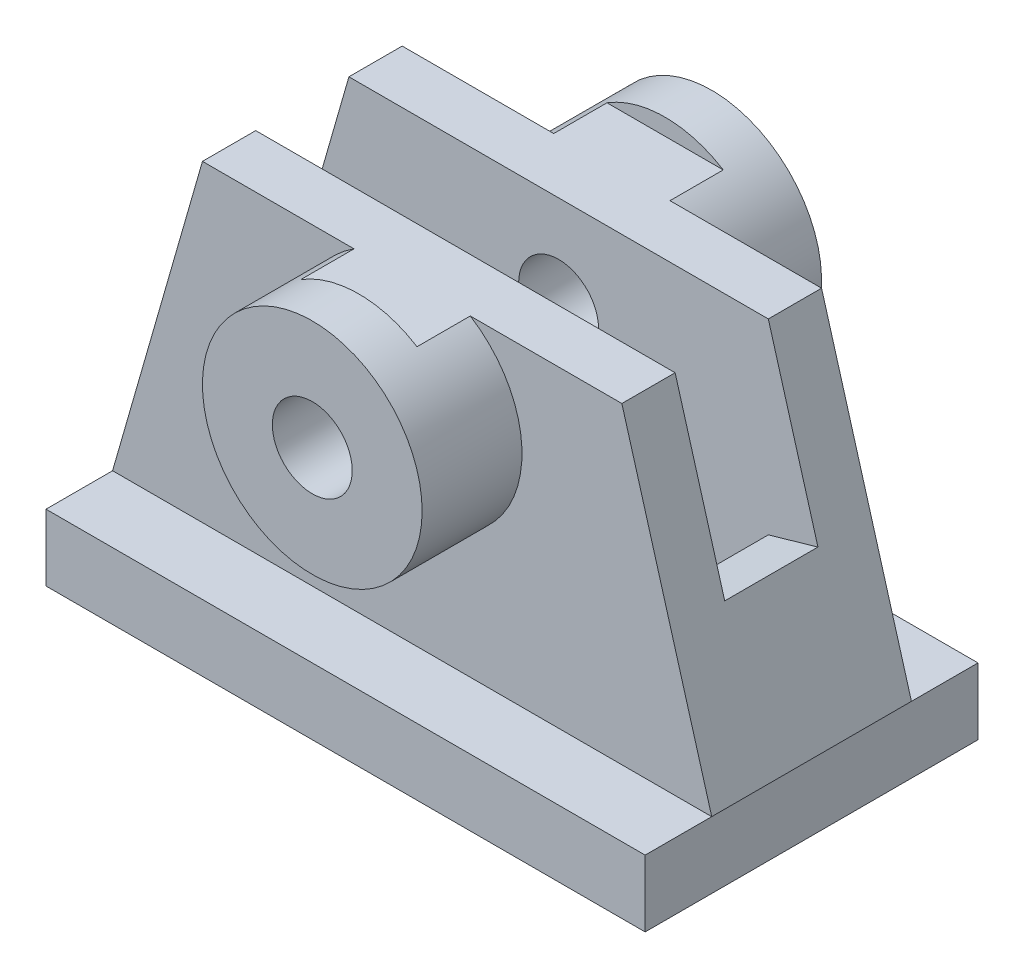
ISO-10303-21;
HEADER;
FILE_DESCRIPTION(('STEP AP214'),'2;1');
FILE_NAME('part.step','',(''),(''),'','','');
FILE_SCHEMA(('AUTOMOTIVE_DESIGN { 1 0 10303 214 1 1 1 1 }'));
ENDSEC;
DATA;
#1=APPLICATION_CONTEXT('core data for automotive mechanical design processes');
#2=APPLICATION_PROTOCOL_DEFINITION('international standard','automotive_design',2000,#1);
#3=PRODUCT_CONTEXT('',#1,'mechanical');
#4=PRODUCT('Part','Part','',(#3));
#5=PRODUCT_RELATED_PRODUCT_CATEGORY('part','',(#4));
#6=PRODUCT_DEFINITION_FORMATION('','',#4);
#7=PRODUCT_DEFINITION_CONTEXT('part definition',#1,'design');
#8=PRODUCT_DEFINITION('design','',#6,#7);
#9=PRODUCT_DEFINITION_SHAPE('','',#8);
#10=(LENGTH_UNIT() NAMED_UNIT(*) SI_UNIT(.MILLI.,.METRE.));
#11=(NAMED_UNIT(*) PLANE_ANGLE_UNIT() SI_UNIT($,.RADIAN.));
#12=(NAMED_UNIT(*) SI_UNIT($,.STERADIAN.) SOLID_ANGLE_UNIT());
#13=UNCERTAINTY_MEASURE_WITH_UNIT(LENGTH_MEASURE(1.E-05),#10,'distance_accuracy_value','');
#14=(GEOMETRIC_REPRESENTATION_CONTEXT(3) GLOBAL_UNCERTAINTY_ASSIGNED_CONTEXT((#13)) GLOBAL_UNIT_ASSIGNED_CONTEXT((#10,
#11,#12)) REPRESENTATION_CONTEXT('',''));
#15=CARTESIAN_POINT('',(0.,0.,0.));
#16=DIRECTION('',(0.,0.,1.));
#17=DIRECTION('',(1.,0.,0.));
#18=AXIS2_PLACEMENT_3D('',#15,#16,#17);
#19=CARTESIAN_POINT('',(0.,43.,-30.));
#20=DIRECTION('',(0.,0.,1.));
#21=DIRECTION('',(1.,0.,0.));
#22=AXIS2_PLACEMENT_3D('',#19,#20,#21);
#23=CYLINDRICAL_SURFACE('',#22,16.5);
#24=CARTESIAN_POINT('',(0.,43.,-30.));
#25=DIRECTION('',(0.,0.,-1.));
#26=DIRECTION('',(-1.,0.,0.));
#27=AXIS2_PLACEMENT_3D('',#24,#25,#26);
#28=CIRCLE('',#27,16.5);
#29=CARTESIAN_POINT('',(-16.5,43.,-30.));
#30=VERTEX_POINT('',#29);
#31=EDGE_CURVE('E334',#30,#30,#28,.T.);
#32=ORIENTED_EDGE('',*,*,#31,.F.);
#33=EDGE_LOOP('',(#32));
#34=FACE_BOUND('',#33,.T.);
#35=DIRECTION('',(0.,0.,-1.));
#36=VECTOR('',#35,1.);
#37=CARTESIAN_POINT('',(-8.73212459828648,57.,195.564259305483));
#38=LINE('',#37,#36);
#39=CARTESIAN_POINT('',(-8.73212459828648,57.,-15.));
#40=VERTEX_POINT('',#39);
#41=CARTESIAN_POINT('',(-8.73212459828648,57.,-23.));
#42=VERTEX_POINT('',#41);
#43=EDGE_CURVE('E177',#40,#42,#38,.T.);
#44=ORIENTED_EDGE('',*,*,#43,.T.);
#45=CARTESIAN_POINT('',(0.,43.,-23.));
#46=DIRECTION('',(0.,0.,-1.));
#47=DIRECTION('',(-1.,0.,0.));
#48=AXIS2_PLACEMENT_3D('',#45,#46,#47);
#49=CIRCLE('',#48,16.5);
#50=CARTESIAN_POINT('',(8.73212459828648,57.,-23.));
#51=VERTEX_POINT('',#50);
#52=EDGE_CURVE('E350',#42,#51,#49,.T.);
#53=ORIENTED_EDGE('',*,*,#52,.T.);
#54=DIRECTION('',(0.,0.,-1.));
#55=VECTOR('',#54,1.);
#56=CARTESIAN_POINT('',(8.73212459828648,57.,195.564259305483));
#57=LINE('',#56,#55);
#58=CARTESIAN_POINT('',(8.73212459828648,57.,-15.));
#59=VERTEX_POINT('',#58);
#60=EDGE_CURVE('E53',#59,#51,#57,.T.);
#61=ORIENTED_EDGE('',*,*,#60,.F.);
#62=CARTESIAN_POINT('',(0.,43.,-15.));
#63=DIRECTION('',(0.,0.,-1.));
#64=DIRECTION('',(-1.,0.,0.));
#65=AXIS2_PLACEMENT_3D('',#62,#63,#64);
#66=CIRCLE('',#65,16.5);
#67=EDGE_CURVE('E50',#40,#59,#66,.F.);
#68=ORIENTED_EDGE('',*,*,#67,.F.);
#69=EDGE_LOOP('',(#44,#53,#61,#68));
#70=FACE_BOUND('',#69,.T.);
#71=ADVANCED_FACE('F39',(#34,#70),#23,.T.);
#72=CARTESIAN_POINT('',(0.,43.,30.));
#73=DIRECTION('',(0.,0.,-1.));
#74=DIRECTION('',(-1.,0.,0.));
#75=AXIS2_PLACEMENT_3D('',#72,#73,#74);
#76=CYLINDRICAL_SURFACE('',#75,16.5);
#77=CARTESIAN_POINT('',(0.,43.,30.));
#78=DIRECTION('',(0.,0.,1.));
#79=DIRECTION('',(1.,0.,0.));
#80=AXIS2_PLACEMENT_3D('',#77,#78,#79);
#81=CIRCLE('',#80,16.5);
#82=CARTESIAN_POINT('',(16.5,43.,30.));
#83=VERTEX_POINT('',#82);
#84=EDGE_CURVE('E337',#83,#83,#81,.T.);
#85=ORIENTED_EDGE('',*,*,#84,.F.);
#86=EDGE_LOOP('',(#85));
#87=FACE_BOUND('',#86,.T.);
#88=DIRECTION('',(0.,0.,1.));
#89=VECTOR('',#88,1.);
#90=CARTESIAN_POINT('',(8.73212459828648,57.,-149.314259305484));
#91=LINE('',#90,#89);
#92=CARTESIAN_POINT('',(8.73212459828648,57.,15.));
#93=VERTEX_POINT('',#92);
#94=CARTESIAN_POINT('',(8.73212459828648,57.,23.));
#95=VERTEX_POINT('',#94);
#96=EDGE_CURVE('E336',#93,#95,#91,.T.);
#97=ORIENTED_EDGE('',*,*,#96,.T.);
#98=CARTESIAN_POINT('',(0.,43.,23.));
#99=DIRECTION('',(0.,0.,1.));
#100=DIRECTION('',(1.,0.,0.));
#101=AXIS2_PLACEMENT_3D('',#98,#99,#100);
#102=CIRCLE('',#101,16.5);
#103=CARTESIAN_POINT('',(-8.73212459828648,57.,23.));
#104=VERTEX_POINT('',#103);
#105=EDGE_CURVE('E187',#95,#104,#102,.T.);
#106=ORIENTED_EDGE('',*,*,#105,.T.);
#107=DIRECTION('',(0.,0.,1.));
#108=VECTOR('',#107,1.);
#109=CARTESIAN_POINT('',(-8.73212459828648,57.,-149.314259305484));
#110=LINE('',#109,#108);
#111=CARTESIAN_POINT('',(-8.73212459828648,57.,15.));
#112=VERTEX_POINT('',#111);
#113=EDGE_CURVE('E64',#112,#104,#110,.T.);
#114=ORIENTED_EDGE('',*,*,#113,.F.);
#115=CARTESIAN_POINT('',(0.,43.,15.));
#116=DIRECTION('',(0.,0.,-1.));
#117=DIRECTION('',(-1.,0.,0.));
#118=AXIS2_PLACEMENT_3D('',#115,#116,#117);
#119=CIRCLE('',#118,16.5);
#120=EDGE_CURVE('E11',#112,#93,#119,.F.);
#121=ORIENTED_EDGE('',*,*,#120,.T.);
#122=EDGE_LOOP('',(#97,#106,#114,#121));
#123=FACE_BOUND('',#122,.T.);
#124=ADVANCED_FACE('F386',(#87,#123),#76,.T.);
#125=CARTESIAN_POINT('',(-31.4970177201008,57.,15.));
#126=DIRECTION('',(0.,-1.,0.));
#127=DIRECTION('',(0.,0.,-1.));
#128=AXIS2_PLACEMENT_3D('',#125,#126,#127);
#129=PLANE('',#128);
#130=DIRECTION('',(0.,0.,-1.));
#131=VECTOR('',#130,1.);
#132=CARTESIAN_POINT('',(31.5029822798992,57.,15.));
#133=LINE('',#132,#131);
#134=CARTESIAN_POINT('',(31.5029822798992,57.,15.));
#135=VERTEX_POINT('',#134);
#136=CARTESIAN_POINT('',(31.5029822798992,57.,7.));
#137=VERTEX_POINT('',#136);
#138=EDGE_CURVE('E214',#135,#137,#133,.T.);
#139=ORIENTED_EDGE('',*,*,#138,.T.);
#140=DIRECTION('',(1.,0.,0.));
#141=VECTOR('',#140,1.);
#142=CARTESIAN_POINT('',(-31.5029822798992,57.,7.));
#143=LINE('',#142,#141);
#144=CARTESIAN_POINT('',(-31.4970177201008,57.,7.));
#145=VERTEX_POINT('',#144);
#146=EDGE_CURVE('E302',#145,#137,#143,.T.);
#147=ORIENTED_EDGE('',*,*,#146,.F.);
#148=DIRECTION('',(0.,0.,-1.));
#149=VECTOR('',#148,1.);
#150=CARTESIAN_POINT('',(-31.4970177201008,57.,15.));
#151=LINE('',#150,#149);
#152=CARTESIAN_POINT('',(-31.4970177201008,57.,15.));
#153=VERTEX_POINT('',#152);
#154=EDGE_CURVE('E211',#153,#145,#151,.T.);
#155=ORIENTED_EDGE('',*,*,#154,.F.);
#156=DIRECTION('',(-1.,0.,0.));
#157=VECTOR('',#156,1.);
#158=CARTESIAN_POINT('',(-31.4970177201008,57.,15.));
#159=LINE('',#158,#157);
#160=EDGE_CURVE('E292',#112,#153,#159,.T.);
#161=ORIENTED_EDGE('',*,*,#160,.F.);
#162=ORIENTED_EDGE('',*,*,#113,.T.);
#163=DIRECTION('',(1.,0.,0.));
#164=VECTOR('',#163,1.);
#165=CARTESIAN_POINT('',(8.73212459828648,57.,23.));
#166=LINE('',#165,#164);
#167=EDGE_CURVE('E344',#104,#95,#166,.T.);
#168=ORIENTED_EDGE('',*,*,#167,.T.);
#169=ORIENTED_EDGE('',*,*,#96,.F.);
#170=EDGE_CURVE('E295',#135,#93,#159,.T.);
#171=ORIENTED_EDGE('',*,*,#170,.F.);
#172=EDGE_LOOP('',(#139,#147,#155,#161,#162,#168,#169,#171));
#173=FACE_BOUND('',#172,.T.);
#174=ADVANCED_FACE('F399',(#173),#129,.F.);
#175=CARTESIAN_POINT('',(0.,10.,0.));
#176=DIRECTION('',(0.,-1.,0.));
#177=DIRECTION('',(0.,0.,-1.));
#178=AXIS2_PLACEMENT_3D('',#175,#176,#177);
#179=PLANE('',#178);
#180=DIRECTION('',(1.,0.,0.));
#181=VECTOR('',#180,1.);
#182=CARTESIAN_POINT('',(-45.,10.,15.));
#183=LINE('',#182,#181);
#184=CARTESIAN_POINT('',(-45.,10.,15.));
#185=VERTEX_POINT('',#184);
#186=CARTESIAN_POINT('',(45.,10.,15.));
#187=VERTEX_POINT('',#186);
#188=EDGE_CURVE('E206',#185,#187,#183,.T.);
#189=ORIENTED_EDGE('',*,*,#188,.F.);
#190=DIRECTION('',(0.,0.,1.));
#191=VECTOR('',#190,1.);
#192=CARTESIAN_POINT('',(-45.,10.,25.));
#193=LINE('',#192,#191);
#194=CARTESIAN_POINT('',(-45.,10.,25.));
#195=VERTEX_POINT('',#194);
#196=EDGE_CURVE('E229',#185,#195,#193,.T.);
#197=ORIENTED_EDGE('',*,*,#196,.T.);
#198=DIRECTION('',(1.,0.,0.));
#199=VECTOR('',#198,1.);
#200=CARTESIAN_POINT('',(-45.,10.,25.));
#201=LINE('',#200,#199);
#202=CARTESIAN_POINT('',(45.,10.,25.));
#203=VERTEX_POINT('',#202);
#204=EDGE_CURVE('E232',#195,#203,#201,.T.);
#205=ORIENTED_EDGE('',*,*,#204,.T.);
#206=DIRECTION('',(0.,0.,-1.));
#207=VECTOR('',#206,1.);
#208=CARTESIAN_POINT('',(45.,10.,25.));
#209=LINE('',#208,#207);
#210=EDGE_CURVE('E225',#203,#187,#209,.T.);
#211=ORIENTED_EDGE('',*,*,#210,.T.);
#212=EDGE_LOOP('',(#189,#197,#205,#211));
#213=FACE_BOUND('',#212,.T.);
#214=ADVANCED_FACE('F567',(#213),#179,.F.);
#215=CARTESIAN_POINT('',(45.,10.,25.));
#216=DIRECTION('',(-1.,0.,0.));
#217=DIRECTION('',(0.,0.,1.));
#218=AXIS2_PLACEMENT_3D('',#215,#216,#217);
#219=PLANE('',#218);
#220=DIRECTION('',(0.,0.,-1.));
#221=VECTOR('',#220,1.);
#222=CARTESIAN_POINT('',(45.,0.,25.));
#223=LINE('',#222,#221);
#224=CARTESIAN_POINT('',(45.,0.,25.));
#225=VERTEX_POINT('',#224);
#226=CARTESIAN_POINT('',(45.,0.,-25.));
#227=VERTEX_POINT('',#226);
#228=EDGE_CURVE('E222',#225,#227,#223,.T.);
#229=ORIENTED_EDGE('',*,*,#228,.T.);
#230=DIRECTION('',(0.,-1.,0.));
#231=VECTOR('',#230,1.);
#232=CARTESIAN_POINT('',(45.,10.,-25.));
#233=LINE('',#232,#231);
#234=CARTESIAN_POINT('',(45.,10.,-25.));
#235=VERTEX_POINT('',#234);
#236=EDGE_CURVE('E248',#235,#227,#233,.T.);
#237=ORIENTED_EDGE('',*,*,#236,.F.);
#238=CARTESIAN_POINT('',(45.,10.,-15.));
#239=VERTEX_POINT('',#238);
#240=EDGE_CURVE('E223',#239,#235,#209,.T.);
#241=ORIENTED_EDGE('',*,*,#240,.F.);
#242=DIRECTION('',(0.,0.,-1.));
#243=VECTOR('',#242,1.);
#244=CARTESIAN_POINT('',(45.,10.,15.));
#245=LINE('',#244,#243);
#246=EDGE_CURVE('E217',#187,#239,#245,.T.);
#247=ORIENTED_EDGE('',*,*,#246,.F.);
#248=ORIENTED_EDGE('',*,*,#210,.F.);
#249=DIRECTION('',(0.,-1.,0.));
#250=VECTOR('',#249,1.);
#251=CARTESIAN_POINT('',(45.,10.,25.));
#252=LINE('',#251,#250);
#253=EDGE_CURVE('E235',#203,#225,#252,.T.);
#254=ORIENTED_EDGE('',*,*,#253,.T.);
#255=EDGE_LOOP('',(#229,#237,#241,#247,#248,#254));
#256=FACE_BOUND('',#255,.T.);
#257=ADVANCED_FACE('F41',(#256),#219,.F.);
#258=CARTESIAN_POINT('',(-45.,10.,-25.));
#259=DIRECTION('',(0.,0.,1.));
#260=DIRECTION('',(1.,0.,0.));
#261=AXIS2_PLACEMENT_3D('',#258,#259,#260);
#262=PLANE('',#261);
#263=DIRECTION('',(-1.,0.,0.));
#264=VECTOR('',#263,1.);
#265=CARTESIAN_POINT('',(-45.,0.,-25.));
#266=LINE('',#265,#264);
#267=CARTESIAN_POINT('',(-45.,0.,-25.));
#268=VERTEX_POINT('',#267);
#269=EDGE_CURVE('E237',#227,#268,#266,.T.);
#270=ORIENTED_EDGE('',*,*,#269,.T.);
#271=DIRECTION('',(0.,-1.,0.));
#272=VECTOR('',#271,1.);
#273=CARTESIAN_POINT('',(-45.,10.,-25.));
#274=LINE('',#273,#272);
#275=CARTESIAN_POINT('',(-45.,10.,-25.));
#276=VERTEX_POINT('',#275);
#277=EDGE_CURVE('E249',#276,#268,#274,.T.);
#278=ORIENTED_EDGE('',*,*,#277,.F.);
#279=DIRECTION('',(-1.,0.,0.));
#280=VECTOR('',#279,1.);
#281=CARTESIAN_POINT('',(-45.,10.,-25.));
#282=LINE('',#281,#280);
#283=EDGE_CURVE('E221',#235,#276,#282,.T.);
#284=ORIENTED_EDGE('',*,*,#283,.F.);
#285=ORIENTED_EDGE('',*,*,#236,.T.);
#286=EDGE_LOOP('',(#270,#278,#284,#285));
#287=FACE_BOUND('',#286,.T.);
#288=ADVANCED_FACE('F446',(#287),#262,.F.);
#289=CARTESIAN_POINT('',(-45.,10.,25.));
#290=DIRECTION('',(1.,0.,0.));
#291=DIRECTION('',(0.,0.,-1.));
#292=AXIS2_PLACEMENT_3D('',#289,#290,#291);
#293=PLANE('',#292);
#294=DIRECTION('',(0.,0.,1.));
#295=VECTOR('',#294,1.);
#296=CARTESIAN_POINT('',(-45.,0.,25.));
#297=LINE('',#296,#295);
#298=CARTESIAN_POINT('',(-45.,0.,25.));
#299=VERTEX_POINT('',#298);
#300=EDGE_CURVE('E236',#268,#299,#297,.T.);
#301=ORIENTED_EDGE('',*,*,#300,.T.);
#302=DIRECTION('',(0.,-1.,0.));
#303=VECTOR('',#302,1.);
#304=CARTESIAN_POINT('',(-45.,10.,25.));
#305=LINE('',#304,#303);
#306=EDGE_CURVE('E241',#195,#299,#305,.T.);
#307=ORIENTED_EDGE('',*,*,#306,.F.);
#308=ORIENTED_EDGE('',*,*,#196,.F.);
#309=DIRECTION('',(0.,0.,-1.));
#310=VECTOR('',#309,1.);
#311=CARTESIAN_POINT('',(-45.,10.,15.));
#312=LINE('',#311,#310);
#313=CARTESIAN_POINT('',(-45.,10.,-15.));
#314=VERTEX_POINT('',#313);
#315=EDGE_CURVE('E210',#185,#314,#312,.T.);
#316=ORIENTED_EDGE('',*,*,#315,.T.);
#317=EDGE_CURVE('E230',#276,#314,#193,.T.);
#318=ORIENTED_EDGE('',*,*,#317,.F.);
#319=ORIENTED_EDGE('',*,*,#277,.T.);
#320=EDGE_LOOP('',(#301,#307,#308,#316,#318,#319));
#321=FACE_BOUND('',#320,.T.);
#322=ADVANCED_FACE('F455',(#321),#293,.F.);
#323=CARTESIAN_POINT('',(-45.,10.,25.));
#324=DIRECTION('',(0.,0.,-1.));
#325=DIRECTION('',(-1.,0.,0.));
#326=AXIS2_PLACEMENT_3D('',#323,#324,#325);
#327=PLANE('',#326);
#328=DIRECTION('',(1.,0.,0.));
#329=VECTOR('',#328,1.);
#330=CARTESIAN_POINT('',(-45.,0.,25.));
#331=LINE('',#330,#329);
#332=EDGE_CURVE('E238',#299,#225,#331,.T.);
#333=ORIENTED_EDGE('',*,*,#332,.T.);
#334=ORIENTED_EDGE('',*,*,#253,.F.);
#335=ORIENTED_EDGE('',*,*,#204,.F.);
#336=ORIENTED_EDGE('',*,*,#306,.T.);
#337=EDGE_LOOP('',(#333,#334,#335,#336));
#338=FACE_BOUND('',#337,.T.);
#339=ADVANCED_FACE('F624',(#338),#327,.F.);
#340=ORIENTED_EDGE('',*,*,#317,.T.);
#341=DIRECTION('',(1.,0.,0.));
#342=VECTOR('',#341,1.);
#343=CARTESIAN_POINT('',(-45.,10.,-15.));
#344=LINE('',#343,#342);
#345=EDGE_CURVE('E203',#314,#239,#344,.T.);
#346=ORIENTED_EDGE('',*,*,#345,.T.);
#347=ORIENTED_EDGE('',*,*,#240,.T.);
#348=ORIENTED_EDGE('',*,*,#283,.T.);
#349=EDGE_LOOP('',(#340,#346,#347,#348));
#350=FACE_BOUND('',#349,.T.);
#351=ADVANCED_FACE('F447',(#350),#179,.F.);
#352=CARTESIAN_POINT('',(0.,0.,0.));
#353=DIRECTION('',(0.,-1.,0.));
#354=DIRECTION('',(0.,0.,-1.));
#355=AXIS2_PLACEMENT_3D('',#352,#353,#354);
#356=PLANE('',#355);
#357=ORIENTED_EDGE('',*,*,#228,.F.);
#358=ORIENTED_EDGE('',*,*,#332,.F.);
#359=ORIENTED_EDGE('',*,*,#300,.F.);
#360=ORIENTED_EDGE('',*,*,#269,.F.);
#361=EDGE_LOOP('',(#357,#358,#359,#360));
#362=FACE_BOUND('',#361,.T.);
#363=ADVANCED_FACE('F597',(#362),#356,.T.);
#364=CARTESIAN_POINT('',(31.5029822798992,57.,15.));
#365=DIRECTION('',(-0.961153336395886,-0.276014970490836,0.));
#366=DIRECTION('',(0.276014970490836,-0.961153336395886,0.));
#367=AXIS2_PLACEMENT_3D('',#364,#365,#366);
#368=PLANE('',#367);
#369=DIRECTION('',(0.,0.,-1.));
#370=VECTOR('',#369,1.);
#371=CARTESIAN_POINT('',(38.9553864831518,31.0488599173111,7.));
#372=LINE('',#371,#370);
#373=CARTESIAN_POINT('',(38.9553864831518,31.0488599173111,7.));
#374=VERTEX_POINT('',#373);
#375=CARTESIAN_POINT('',(38.9553864831518,31.0488599173111,-7.));
#376=VERTEX_POINT('',#375);
#377=EDGE_CURVE('E316',#374,#376,#372,.T.);
#378=ORIENTED_EDGE('',*,*,#377,.F.);
#379=DIRECTION('',(0.276014970490836,-0.961153336395886,0.));
#380=VECTOR('',#379,1.);
#381=CARTESIAN_POINT('',(31.5029822798992,57.,7.));
#382=LINE('',#381,#380);
#383=EDGE_CURVE('E318',#137,#374,#382,.T.);
#384=ORIENTED_EDGE('',*,*,#383,.F.);
#385=ORIENTED_EDGE('',*,*,#138,.F.);
#386=DIRECTION('',(-0.276014970490836,0.961153336395886,0.));
#387=VECTOR('',#386,1.);
#388=CARTESIAN_POINT('',(31.5029822798992,57.,15.));
#389=LINE('',#388,#387);
#390=EDGE_CURVE('E286',#187,#135,#389,.T.);
#391=ORIENTED_EDGE('',*,*,#390,.F.);
#392=ORIENTED_EDGE('',*,*,#246,.T.);
#393=DIRECTION('',(-0.276014970490836,0.961153336395886,0.));
#394=VECTOR('',#393,1.);
#395=CARTESIAN_POINT('',(31.5029822798992,57.,-15.));
#396=LINE('',#395,#394);
#397=CARTESIAN_POINT('',(31.5029822798992,57.,-15.));
#398=VERTEX_POINT('',#397);
#399=EDGE_CURVE('E196',#239,#398,#396,.T.);
#400=ORIENTED_EDGE('',*,*,#399,.T.);
#401=CARTESIAN_POINT('',(31.5029822798992,57.,-7.));
#402=VERTEX_POINT('',#401);
#403=EDGE_CURVE('E212',#402,#398,#133,.T.);
#404=ORIENTED_EDGE('',*,*,#403,.F.);
#405=DIRECTION('',(-0.276014970490836,0.961153336395886,0.));
#406=VECTOR('',#405,1.);
#407=CARTESIAN_POINT('',(31.5029822798992,57.,-7.));
#408=LINE('',#407,#406);
#409=EDGE_CURVE('E311',#376,#402,#408,.T.);
#410=ORIENTED_EDGE('',*,*,#409,.F.);
#411=EDGE_LOOP('',(#378,#384,#385,#391,#392,#400,#404,#410));
#412=FACE_BOUND('',#411,.T.);
#413=ADVANCED_FACE('F436',(#412),#368,.F.);
#414=CARTESIAN_POINT('',(-31.4970177201008,57.,-7.));
#415=VERTEX_POINT('',#414);
#416=CARTESIAN_POINT('',(-31.4970177201008,57.,-15.));
#417=VERTEX_POINT('',#416);
#418=EDGE_CURVE('E207',#415,#417,#151,.T.);
#419=ORIENTED_EDGE('',*,*,#418,.F.);
#420=DIRECTION('',(-1.,0.,0.));
#421=VECTOR('',#420,1.);
#422=CARTESIAN_POINT('',(-31.5029822798992,57.,-7.));
#423=LINE('',#422,#421);
#424=EDGE_CURVE('E303',#402,#415,#423,.T.);
#425=ORIENTED_EDGE('',*,*,#424,.F.);
#426=ORIENTED_EDGE('',*,*,#403,.T.);
#427=DIRECTION('',(-1.,0.,0.));
#428=VECTOR('',#427,1.);
#429=CARTESIAN_POINT('',(-31.4970177201008,57.,-15.));
#430=LINE('',#429,#428);
#431=EDGE_CURVE('E197',#398,#59,#430,.T.);
#432=ORIENTED_EDGE('',*,*,#431,.T.);
#433=ORIENTED_EDGE('',*,*,#60,.T.);
#434=DIRECTION('',(-1.,0.,0.));
#435=VECTOR('',#434,1.);
#436=CARTESIAN_POINT('',(-8.73212459828648,57.,-23.));
#437=LINE('',#436,#435);
#438=EDGE_CURVE('E181',#51,#42,#437,.T.);
#439=ORIENTED_EDGE('',*,*,#438,.T.);
#440=ORIENTED_EDGE('',*,*,#43,.F.);
#441=EDGE_CURVE('E182',#40,#417,#430,.T.);
#442=ORIENTED_EDGE('',*,*,#441,.T.);
#443=EDGE_LOOP('',(#419,#425,#426,#432,#433,#439,#440,#442));
#444=FACE_BOUND('',#443,.T.);
#445=ADVANCED_FACE('F176',(#444),#129,.F.);
#446=CARTESIAN_POINT('',(-31.4970177201008,57.,15.));
#447=DIRECTION('',(0.961120971624267,-0.276127647844297,0.));
#448=DIRECTION('',(0.276127647844297,0.961120971624267,0.));
#449=AXIS2_PLACEMENT_3D('',#446,#447,#448);
#450=PLANE('',#449);
#451=DIRECTION('',(0.,0.,1.));
#452=VECTOR('',#451,1.);
#453=CARTESIAN_POINT('',(-38.9584287716952,31.0289728479483,-7.));
#454=LINE('',#453,#452);
#455=CARTESIAN_POINT('',(-38.9584287716952,31.0289728479483,-7.));
#456=VERTEX_POINT('',#455);
#457=CARTESIAN_POINT('',(-38.9584287716952,31.0289728479483,7.));
#458=VERTEX_POINT('',#457);
#459=EDGE_CURVE('E327',#456,#458,#454,.T.);
#460=ORIENTED_EDGE('',*,*,#459,.F.);
#461=DIRECTION('',(0.276127647844297,0.961120971624267,0.));
#462=VECTOR('',#461,1.);
#463=CARTESIAN_POINT('',(-31.4970177201008,57.,-7.));
#464=LINE('',#463,#462);
#465=EDGE_CURVE('E251',#456,#415,#464,.T.);
#466=ORIENTED_EDGE('',*,*,#465,.T.);
#467=ORIENTED_EDGE('',*,*,#418,.T.);
#468=DIRECTION('',(-0.276127647844297,-0.961120971624267,0.));
#469=VECTOR('',#468,1.);
#470=CARTESIAN_POINT('',(-31.4970177201008,57.,-15.));
#471=LINE('',#470,#469);
#472=EDGE_CURVE('E198',#417,#314,#471,.T.);
#473=ORIENTED_EDGE('',*,*,#472,.T.);
#474=ORIENTED_EDGE('',*,*,#315,.F.);
#475=DIRECTION('',(-0.276127647844297,-0.961120971624267,0.));
#476=VECTOR('',#475,1.);
#477=CARTESIAN_POINT('',(-31.4970177201008,57.,15.));
#478=LINE('',#477,#476);
#479=EDGE_CURVE('E209',#153,#185,#478,.T.);
#480=ORIENTED_EDGE('',*,*,#479,.F.);
#481=ORIENTED_EDGE('',*,*,#154,.T.);
#482=DIRECTION('',(-0.276127647844297,-0.961120971624267,0.));
#483=VECTOR('',#482,1.);
#484=CARTESIAN_POINT('',(-31.4970177201008,57.,7.));
#485=LINE('',#484,#483);
#486=EDGE_CURVE('E258',#145,#458,#485,.T.);
#487=ORIENTED_EDGE('',*,*,#486,.T.);
#488=EDGE_LOOP('',(#460,#466,#467,#473,#474,#480,#481,#487));
#489=FACE_BOUND('',#488,.T.);
#490=ADVANCED_FACE('F430',(#489),#450,.F.);
#491=CARTESIAN_POINT('',(0.,0.,15.));
#492=DIRECTION('',(0.,0.,-1.));
#493=DIRECTION('',(-1.,0.,0.));
#494=AXIS2_PLACEMENT_3D('',#491,#492,#493);
#495=PLANE('',#494);
#496=ORIENTED_EDGE('',*,*,#120,.F.);
#497=ORIENTED_EDGE('',*,*,#160,.T.);
#498=ORIENTED_EDGE('',*,*,#479,.T.);
#499=ORIENTED_EDGE('',*,*,#188,.T.);
#500=ORIENTED_EDGE('',*,*,#390,.T.);
#501=ORIENTED_EDGE('',*,*,#170,.T.);
#502=EDGE_LOOP('',(#496,#497,#498,#499,#500,#501));
#503=FACE_BOUND('',#502,.T.);
#504=ADVANCED_FACE('F416',(#503),#495,.F.);
#505=CARTESIAN_POINT('',(0.,0.,-15.));
#506=DIRECTION('',(0.,0.,-1.));
#507=DIRECTION('',(-1.,0.,0.));
#508=AXIS2_PLACEMENT_3D('',#505,#506,#507);
#509=PLANE('',#508);
#510=ORIENTED_EDGE('',*,*,#441,.F.);
#511=ORIENTED_EDGE('',*,*,#67,.T.);
#512=ORIENTED_EDGE('',*,*,#431,.F.);
#513=ORIENTED_EDGE('',*,*,#399,.F.);
#514=ORIENTED_EDGE('',*,*,#345,.F.);
#515=ORIENTED_EDGE('',*,*,#472,.F.);
#516=EDGE_LOOP('',(#510,#511,#512,#513,#514,#515));
#517=FACE_BOUND('',#516,.T.);
#518=ADVANCED_FACE('F195',(#517),#509,.T.);
#519=CARTESIAN_POINT('',(-31.5029822798992,10.,7.));
#520=DIRECTION('',(0.,0.,1.));
#521=DIRECTION('',(1.,0.,0.));
#522=AXIS2_PLACEMENT_3D('',#519,#520,#521);
#523=PLANE('',#522);
#524=CARTESIAN_POINT('',(0.,43.,7.));
#525=DIRECTION('',(0.,0.,1.));
#526=DIRECTION('',(1.,0.,0.));
#527=AXIS2_PLACEMENT_3D('',#524,#525,#526);
#528=CIRCLE('',#527,6.);
#529=CARTESIAN_POINT('',(6.,43.,7.));
#530=VERTEX_POINT('',#529);
#531=EDGE_CURVE('E346',#530,#530,#528,.T.);
#532=ORIENTED_EDGE('',*,*,#531,.T.);
#533=EDGE_LOOP('',(#532));
#534=FACE_BOUND('',#533,.T.);
#535=DIRECTION('',(-0.961120971624267,0.276127647844297,0.));
#536=VECTOR('',#535,1.);
#537=CARTESIAN_POINT('',(-29.3472190554525,28.2676963695053,7.));
#538=LINE('',#537,#536);
#539=CARTESIAN_POINT('',(-31.5029822798992,28.8870417443853,7.));
#540=VERTEX_POINT('',#539);
#541=EDGE_CURVE('E322',#540,#458,#538,.T.);
#542=ORIENTED_EDGE('',*,*,#541,.T.);
#543=ORIENTED_EDGE('',*,*,#486,.F.);
#544=ORIENTED_EDGE('',*,*,#146,.T.);
#545=ORIENTED_EDGE('',*,*,#383,.T.);
#546=DIRECTION('',(0.961153336395886,0.276014970490836,0.));
#547=VECTOR('',#546,1.);
#548=CARTESIAN_POINT('',(29.3438531191929,28.2887102124027,7.));
#549=LINE('',#548,#547);
#550=CARTESIAN_POINT('',(31.5029822798992,28.9087486069142,7.));
#551=VERTEX_POINT('',#550);
#552=EDGE_CURVE('E313',#551,#374,#549,.T.);
#553=ORIENTED_EDGE('',*,*,#552,.F.);
#554=DIRECTION('',(0.,1.,0.));
#555=VECTOR('',#554,1.);
#556=CARTESIAN_POINT('',(31.5029822798992,10.,7.));
#557=LINE('',#556,#555);
#558=CARTESIAN_POINT('',(31.5029822798992,10.,7.));
#559=VERTEX_POINT('',#558);
#560=EDGE_CURVE('E266',#559,#551,#557,.T.);
#561=ORIENTED_EDGE('',*,*,#560,.F.);
#562=DIRECTION('',(1.,0.,0.));
#563=VECTOR('',#562,1.);
#564=CARTESIAN_POINT('',(-31.5029822798992,10.,7.));
#565=LINE('',#564,#563);
#566=CARTESIAN_POINT('',(-31.5029822798992,10.,7.));
#567=VERTEX_POINT('',#566);
#568=EDGE_CURVE('E280',#567,#559,#565,.T.);
#569=ORIENTED_EDGE('',*,*,#568,.F.);
#570=DIRECTION('',(0.,1.,0.));
#571=VECTOR('',#570,1.);
#572=CARTESIAN_POINT('',(-31.5029822798992,10.,7.));
#573=LINE('',#572,#571);
#574=EDGE_CURVE('E278',#567,#540,#573,.T.);
#575=ORIENTED_EDGE('',*,*,#574,.T.);
#576=EDGE_LOOP('',(#542,#543,#544,#545,#553,#561,#569,#575));
#577=FACE_BOUND('',#576,.T.);
#578=ADVANCED_FACE('F384',(#534,#577),#523,.F.);
#579=CARTESIAN_POINT('',(-31.5029822798992,10.,7.));
#580=DIRECTION('',(-1.,0.,0.));
#581=DIRECTION('',(0.,0.,1.));
#582=AXIS2_PLACEMENT_3D('',#579,#580,#581);
#583=PLANE('',#582);
#584=DIRECTION('',(0.,1.,0.));
#585=VECTOR('',#584,1.);
#586=CARTESIAN_POINT('',(-31.5029822798992,10.,-7.));
#587=LINE('',#586,#585);
#588=CARTESIAN_POINT('',(-31.5029822798992,10.,-7.));
#589=VERTEX_POINT('',#588);
#590=CARTESIAN_POINT('',(-31.5029822798992,28.8870417443853,-7.));
#591=VERTEX_POINT('',#590);
#592=EDGE_CURVE('E277',#589,#591,#587,.T.);
#593=ORIENTED_EDGE('',*,*,#592,.T.);
#594=DIRECTION('',(0.,0.,1.));
#595=VECTOR('',#594,1.);
#596=CARTESIAN_POINT('',(-31.5029822798992,28.8870417443853,7.));
#597=LINE('',#596,#595);
#598=EDGE_CURVE('E321',#591,#540,#597,.T.);
#599=ORIENTED_EDGE('',*,*,#598,.T.);
#600=ORIENTED_EDGE('',*,*,#574,.F.);
#601=DIRECTION('',(0.,0.,1.));
#602=VECTOR('',#601,1.);
#603=CARTESIAN_POINT('',(-31.5029822798992,10.,7.));
#604=LINE('',#603,#602);
#605=EDGE_CURVE('E285',#589,#567,#604,.T.);
#606=ORIENTED_EDGE('',*,*,#605,.F.);
#607=EDGE_LOOP('',(#593,#599,#600,#606));
#608=FACE_BOUND('',#607,.T.);
#609=ADVANCED_FACE('F374',(#608),#583,.F.);
#610=CARTESIAN_POINT('',(-31.5029822798992,10.,-7.));
#611=DIRECTION('',(0.,0.,-1.));
#612=DIRECTION('',(-1.,0.,0.));
#613=AXIS2_PLACEMENT_3D('',#610,#611,#612);
#614=PLANE('',#613);
#615=CARTESIAN_POINT('',(0.,43.,-7.));
#616=DIRECTION('',(0.,0.,-1.));
#617=DIRECTION('',(-1.,0.,0.));
#618=AXIS2_PLACEMENT_3D('',#615,#616,#617);
#619=CIRCLE('',#618,6.);
#620=CARTESIAN_POINT('',(-6.,43.,-7.));
#621=VERTEX_POINT('',#620);
#622=EDGE_CURVE('E351',#621,#621,#619,.T.);
#623=ORIENTED_EDGE('',*,*,#622,.T.);
#624=EDGE_LOOP('',(#623));
#625=FACE_BOUND('',#624,.T.);
#626=ORIENTED_EDGE('',*,*,#465,.F.);
#627=DIRECTION('',(-0.961120971624267,0.276127647844297,0.));
#628=VECTOR('',#627,1.);
#629=CARTESIAN_POINT('',(-29.3472190554525,28.2676963695053,-7.));
#630=LINE('',#629,#628);
#631=EDGE_CURVE('E324',#591,#456,#630,.T.);
#632=ORIENTED_EDGE('',*,*,#631,.F.);
#633=ORIENTED_EDGE('',*,*,#592,.F.);
#634=DIRECTION('',(-1.,0.,0.));
#635=VECTOR('',#634,1.);
#636=CARTESIAN_POINT('',(-31.5029822798992,10.,-7.));
#637=LINE('',#636,#635);
#638=CARTESIAN_POINT('',(31.5029822798992,10.,-7.));
#639=VERTEX_POINT('',#638);
#640=EDGE_CURVE('E273',#639,#589,#637,.T.);
#641=ORIENTED_EDGE('',*,*,#640,.F.);
#642=DIRECTION('',(0.,1.,0.));
#643=VECTOR('',#642,1.);
#644=CARTESIAN_POINT('',(31.5029822798992,10.,-7.));
#645=LINE('',#644,#643);
#646=CARTESIAN_POINT('',(31.5029822798992,28.9087486069142,-7.));
#647=VERTEX_POINT('',#646);
#648=EDGE_CURVE('E262',#639,#647,#645,.T.);
#649=ORIENTED_EDGE('',*,*,#648,.T.);
#650=DIRECTION('',(0.961153336395886,0.276014970490836,0.));
#651=VECTOR('',#650,1.);
#652=CARTESIAN_POINT('',(29.3438531191929,28.2887102124027,-7.));
#653=LINE('',#652,#651);
#654=EDGE_CURVE('E271',#647,#376,#653,.T.);
#655=ORIENTED_EDGE('',*,*,#654,.T.);
#656=ORIENTED_EDGE('',*,*,#409,.T.);
#657=ORIENTED_EDGE('',*,*,#424,.T.);
#658=EDGE_LOOP('',(#626,#632,#633,#641,#649,#655,#656,#657));
#659=FACE_BOUND('',#658,.T.);
#660=ADVANCED_FACE('F269',(#625,#659),#614,.F.);
#661=CARTESIAN_POINT('',(31.5029822798992,10.,7.));
#662=DIRECTION('',(1.,0.,0.));
#663=DIRECTION('',(0.,0.,-1.));
#664=AXIS2_PLACEMENT_3D('',#661,#662,#663);
#665=PLANE('',#664);
#666=ORIENTED_EDGE('',*,*,#560,.T.);
#667=DIRECTION('',(0.,0.,-1.));
#668=VECTOR('',#667,1.);
#669=CARTESIAN_POINT('',(31.5029822798992,28.9087486069142,7.));
#670=LINE('',#669,#668);
#671=EDGE_CURVE('E192',#551,#647,#670,.T.);
#672=ORIENTED_EDGE('',*,*,#671,.T.);
#673=ORIENTED_EDGE('',*,*,#648,.F.);
#674=DIRECTION('',(0.,0.,-1.));
#675=VECTOR('',#674,1.);
#676=CARTESIAN_POINT('',(31.5029822798992,10.,7.));
#677=LINE('',#676,#675);
#678=EDGE_CURVE('E301',#559,#639,#677,.T.);
#679=ORIENTED_EDGE('',*,*,#678,.F.);
#680=EDGE_LOOP('',(#666,#672,#673,#679));
#681=FACE_BOUND('',#680,.T.);
#682=ADVANCED_FACE('F265',(#681),#665,.F.);
#683=CARTESIAN_POINT('',(0.,10.,0.));
#684=DIRECTION('',(0.,-1.,0.));
#685=DIRECTION('',(0.,0.,-1.));
#686=AXIS2_PLACEMENT_3D('',#683,#684,#685);
#687=PLANE('',#686);
#688=ORIENTED_EDGE('',*,*,#678,.T.);
#689=ORIENTED_EDGE('',*,*,#640,.T.);
#690=ORIENTED_EDGE('',*,*,#605,.T.);
#691=ORIENTED_EDGE('',*,*,#568,.T.);
#692=EDGE_LOOP('',(#688,#689,#690,#691));
#693=FACE_BOUND('',#692,.T.);
#694=ADVANCED_FACE('F385',(#693),#687,.F.);
#695=CARTESIAN_POINT('',(29.3438531191929,28.2887102124027,7.));
#696=DIRECTION('',(0.276014970490836,-0.961153336395886,0.));
#697=DIRECTION('',(0.961153336395886,0.276014970490836,0.));
#698=AXIS2_PLACEMENT_3D('',#695,#696,#697);
#699=PLANE('',#698);
#700=ORIENTED_EDGE('',*,*,#552,.T.);
#701=ORIENTED_EDGE('',*,*,#377,.T.);
#702=ORIENTED_EDGE('',*,*,#654,.F.);
#703=ORIENTED_EDGE('',*,*,#671,.F.);
#704=EDGE_LOOP('',(#700,#701,#702,#703));
#705=FACE_BOUND('',#704,.T.);
#706=ADVANCED_FACE('F407',(#705),#699,.F.);
#707=CARTESIAN_POINT('',(-29.3472190554525,28.2676963695053,-7.));
#708=DIRECTION('',(-0.276127647844297,-0.961120971624267,0.));
#709=DIRECTION('',(0.961120971624268,-0.276127647844297,0.));
#710=AXIS2_PLACEMENT_3D('',#707,#708,#709);
#711=PLANE('',#710);
#712=ORIENTED_EDGE('',*,*,#631,.T.);
#713=ORIENTED_EDGE('',*,*,#459,.T.);
#714=ORIENTED_EDGE('',*,*,#541,.F.);
#715=ORIENTED_EDGE('',*,*,#598,.F.);
#716=EDGE_LOOP('',(#712,#713,#714,#715));
#717=FACE_BOUND('',#716,.T.);
#718=ADVANCED_FACE('F401',(#717),#711,.F.);
#719=CARTESIAN_POINT('',(0.,43.,-30.));
#720=DIRECTION('',(0.,0.,-1.));
#721=DIRECTION('',(-1.,0.,0.));
#722=AXIS2_PLACEMENT_3D('',#719,#720,#721);
#723=PLANE('',#722);
#724=CARTESIAN_POINT('',(0.,43.,-30.));
#725=DIRECTION('',(0.,0.,1.));
#726=DIRECTION('',(1.,0.,0.));
#727=AXIS2_PLACEMENT_3D('',#724,#725,#726);
#728=CIRCLE('',#727,6.);
#729=CARTESIAN_POINT('',(6.,43.,-30.));
#730=VERTEX_POINT('',#729);
#731=EDGE_CURVE('E359',#730,#730,#728,.T.);
#732=ORIENTED_EDGE('',*,*,#731,.T.);
#733=EDGE_LOOP('',(#732));
#734=FACE_BOUND('',#733,.T.);
#735=ORIENTED_EDGE('',*,*,#31,.T.);
#736=EDGE_LOOP('',(#735));
#737=FACE_BOUND('',#736,.T.);
#738=ADVANCED_FACE('F365',(#734,#737),#723,.T.);
#739=CARTESIAN_POINT('',(0.,43.,30.));
#740=DIRECTION('',(0.,0.,1.));
#741=DIRECTION('',(1.,0.,0.));
#742=AXIS2_PLACEMENT_3D('',#739,#740,#741);
#743=PLANE('',#742);
#744=CARTESIAN_POINT('',(0.,43.,30.));
#745=DIRECTION('',(0.,0.,1.));
#746=DIRECTION('',(1.,0.,0.));
#747=AXIS2_PLACEMENT_3D('',#744,#745,#746);
#748=CIRCLE('',#747,6.);
#749=CARTESIAN_POINT('',(6.,43.,30.));
#750=VERTEX_POINT('',#749);
#751=EDGE_CURVE('E360',#750,#750,#748,.T.);
#752=ORIENTED_EDGE('',*,*,#751,.F.);
#753=EDGE_LOOP('',(#752));
#754=FACE_BOUND('',#753,.T.);
#755=ORIENTED_EDGE('',*,*,#84,.T.);
#756=EDGE_LOOP('',(#755));
#757=FACE_BOUND('',#756,.T.);
#758=ADVANCED_FACE('F461',(#754,#757),#743,.T.);
#759=CARTESIAN_POINT('',(0.,43.,23.));
#760=DIRECTION('',(0.,0.,1.));
#761=DIRECTION('',(1.,0.,0.));
#762=AXIS2_PLACEMENT_3D('',#759,#760,#761);
#763=PLANE('',#762);
#764=ORIENTED_EDGE('',*,*,#105,.F.);
#765=ORIENTED_EDGE('',*,*,#167,.F.);
#766=EDGE_LOOP('',(#764,#765));
#767=FACE_BOUND('',#766,.T.);
#768=ADVANCED_FACE('F464',(#767),#763,.F.);
#769=CARTESIAN_POINT('',(0.,43.,-23.));
#770=DIRECTION('',(0.,0.,-1.));
#771=DIRECTION('',(-1.,0.,0.));
#772=AXIS2_PLACEMENT_3D('',#769,#770,#771);
#773=PLANE('',#772);
#774=ORIENTED_EDGE('',*,*,#52,.F.);
#775=ORIENTED_EDGE('',*,*,#438,.F.);
#776=EDGE_LOOP('',(#774,#775));
#777=FACE_BOUND('',#776,.T.);
#778=ADVANCED_FACE('F465',(#777),#773,.F.);
#779=CARTESIAN_POINT('',(0.,43.,-30.));
#780=DIRECTION('',(0.,0.,1.));
#781=DIRECTION('',(1.,0.,0.));
#782=AXIS2_PLACEMENT_3D('',#779,#780,#781);
#783=CYLINDRICAL_SURFACE('',#782,6.);
#784=ORIENTED_EDGE('',*,*,#751,.T.);
#785=EDGE_LOOP('',(#784));
#786=FACE_BOUND('',#785,.T.);
#787=ORIENTED_EDGE('',*,*,#531,.F.);
#788=EDGE_LOOP('',(#787));
#789=FACE_BOUND('',#788,.T.);
#790=ADVANCED_FACE('F367',(#786,#789),#783,.F.);
#791=ORIENTED_EDGE('',*,*,#731,.F.);
#792=EDGE_LOOP('',(#791));
#793=FACE_BOUND('',#792,.T.);
#794=ORIENTED_EDGE('',*,*,#622,.F.);
#795=EDGE_LOOP('',(#794));
#796=FACE_BOUND('',#795,.T.);
#797=ADVANCED_FACE('F370',(#793,#796),#783,.F.);
#798=CLOSED_SHELL('',(#71,#124,#174,#214,#257,#288,#322,#339,#351,#363,#413,#445,#490,#504,#518,
#578,#609,#660,#682,#694,#706,#718,#738,#758,#768,#778,#790,#797));
#799=MANIFOLD_SOLID_BREP('B2',#798);
#800=ADVANCED_BREP_SHAPE_REPRESENTATION('',(#18,#799),#14);
#801=SHAPE_DEFINITION_REPRESENTATION(#9,#800);
ENDSEC;
END-ISO-10303-21;
